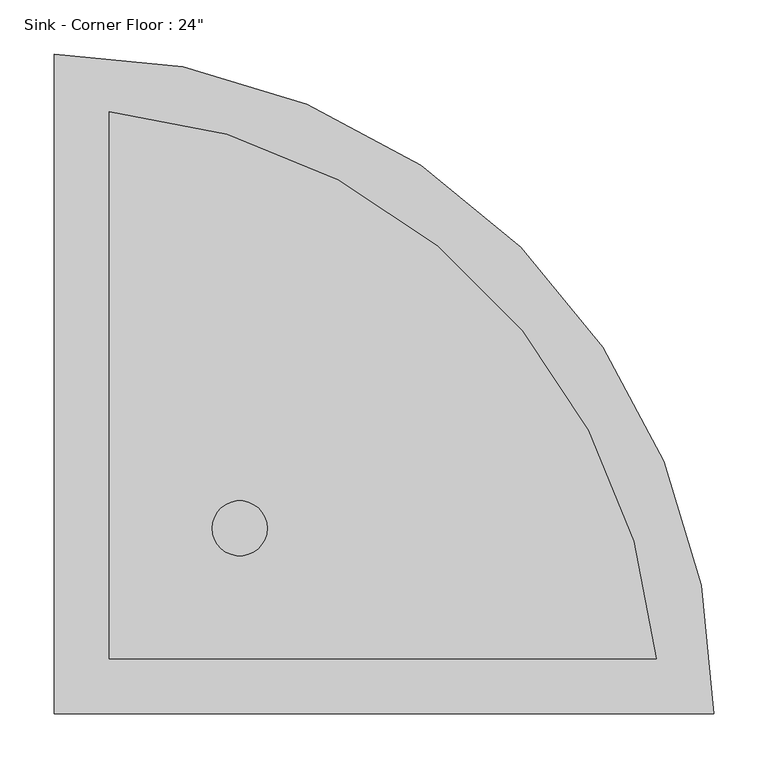
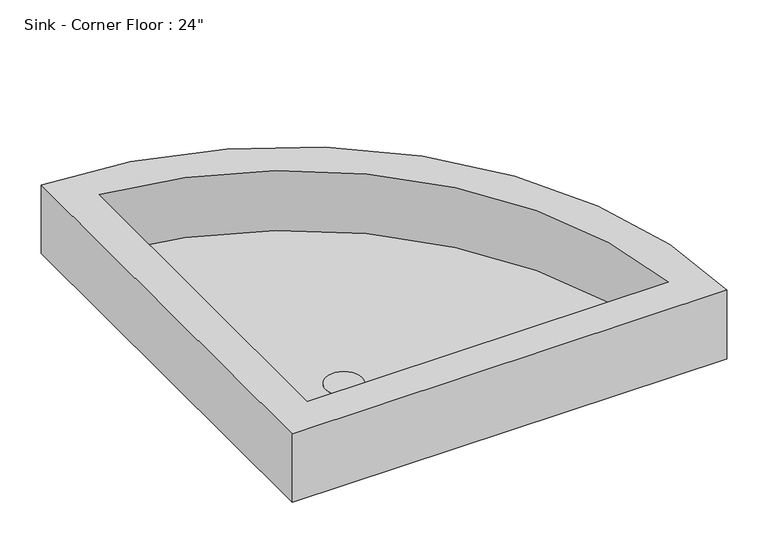
"""IFC4 building model written with IfcOpenShell, lengths in millimetres: flow terminal geometry."""

from ifc_helpers import new_model, si_unit, point, frame, frame_2d, origin, origin_with_axes, place, context, project, spatial, polyline, circle_curve, trimmed, segment, composite_curve, outline, extrude, source, transform, mapped, element, save
from ifc_brep_helpers import plane_surface, cylinder_surface, revolved_surface, advanced_brep


def flow_terminal_bd5cdcf8(model_context):
    return source(origin(), model_context, "Body", "SolidModel", [
        extrude(outline(composite_curve([segment(trimmed(circle_curve(frame_2d((171.45, 171.45)), 25.4), [point((146.05, 171.45))], [point((196.85, 171.45))], False, "CARTESIAN"), True, "CONTINUOUS"), segment(trimmed(circle_curve(frame_2d((171.45, 171.45)), 25.4), [point((196.85, 171.45))], [point((146.05, 171.45))], False, "CARTESIAN"), True, "CONTINUOUS")], self_intersect=False)), origin_with_axes(), (0.0, 0.0, 1.0), 12.7),
        advanced_brep(
        [(0.0, 0.0, 101.6), (609.6, 0.0, 101.6), (0.0, 609.6, 101.6), (556.4861184, 50.8, 101.6), (50.8, 50.8, 101.6), (50.8, 556.4861184, 101.6), (0.0, 0.0, 0.0), (0.0, 609.6, 0.0), (609.6, 0.0, 0.0), (50.8, 50.8, 12.7), (556.4861184, 50.8, 12.7), (50.8, 556.4861184, 12.7)],
        [
            (0, 1),
            (1, 2, circle_curve(frame((0.0, 0.0, 101.6), z_axis=(0.0, 0.0, 1.0), x_axis=(1.0, 0.0, 0.0)), 609.6)),
            (2, 0),
            (3, 4),
            (4, 5),
            (5, 3, circle_curve(frame((0.0, 0.0, 101.6), z_axis=(0.0, 0.0, -1.0), x_axis=(1.0, 0.0, 0.0)), 558.8)),
            (6, 7),
            (7, 8, circle_curve(frame((0.0, 0.0, 0.0), z_axis=(0.0, 0.0, -1.0), x_axis=(1.0, 0.0, 0.0)), 609.6)),
            (8, 6),
            (0, 6),
            (8, 1),
            (7, 2),
            (9, 10),
            (10, 11, circle_curve(frame((0.0, 0.0, 12.7), z_axis=(0.0, 0.0, 1.0), x_axis=(1.0, 0.0, 0.0)), 558.8)),
            (11, 9),
            (9, 4),
            (3, 10),
            (5, 11),
        ],
        [
            plane_surface(frame((0.0, 0.0, 101.6), z_axis=(0.0, 0.0, 1.0), x_axis=(1.0, 0.0, 0.0))),
            plane_surface(frame((0.0, 0.0, 0.0), z_axis=(0.0, 0.0, -1.0), x_axis=(-1.0, 0.0, 0.0))),
            plane_surface(frame((0.0, 0.0, 101.6), z_axis=(0.0, -1.0, 0.0), x_axis=(0.0, 0.0, -1.0))),
            cylinder_surface(origin_with_axes(), 609.6),
            plane_surface(frame((0.0, 609.6, 101.6), z_axis=(-1.0, 0.0, 0.0), x_axis=(0.0, 0.0, -1.0))),
            plane_surface(frame((50.8, 50.8, 12.7), z_axis=(0.0, 0.0, 1.0), x_axis=(-1.0, 0.0, 0.0))),
            plane_surface(frame((50.8, 50.8, 101.6), z_axis=(0.0, 1.0, 0.0), x_axis=(0.0, 0.0, -1.0))),
            revolved_surface(polyline([(558.8, 0.0, 101.6), (558.8, 0.0, 12.7)]), (0.0, 0.0, 12.7), (0.0, 0.0, 1.0)),
            plane_surface(frame((50.8, 556.4861184, 101.6), z_axis=(1.0, 0.0, 0.0), x_axis=(0.0, 0.0, -1.0))),
        ],
        [
            (0, [[1, 2, 3], [4, 5, 6]]),
            (1, [[7, 8, 9]]),
            (2, [[-1, 10, -9, 11]]),
            (3, [[-2, -11, -8, 12]]),
            (4, [[-3, -12, -7, -10]]),
            (5, [[13, 14, 15]]),
            (6, [[-13, 16, -4, 17]]),
            (7, [[-14, -17, -6, 18]]),
            (8, [[-15, -18, -5, -16]]),
        ],
    ),
    ])


if __name__ == "__main__":
    model = new_model("IFC4")
    model_context = context("Model", 3, world=origin())
    ifc_project = project(units=[si_unit("LENGTHUNIT", "METRE", prefix="MILLI")], contexts=[model_context])
    site = spatial("IfcSite", under=ifc_project)
    building = spatial("IfcBuilding", under=site)
    placement = place(None, origin())
    flow_terminal_shape = flow_terminal_bd5cdcf8(model_context)
    element("IfcFlowTerminal", 1, ObjectType="Sink - Corner Floor : 24\"", at=placement, inside=building, context=model_context, shape_type="MappedRepresentation", body=[
        mapped(flow_terminal_shape, transform((0.0, 0.0, 0.0), x_axis=(1.0, 0.0, 0.0), y_axis=(0.0, 1.0, 0.0), z_axis=(0.0, 0.0, 1.0))),
    ])
    save(model, "model.ifc")

# Revit data of these elements
# Type "Sink - Corner Floor : 24\""
#   WFU = 2
#   Sink Radius = 2' - 0"
#   Sink Depth = 0' - 3 1/2"
#   Sanitary Radius = 3/4"
#   Sanitary Diameter = 1 1/2"
#   Radius 1 = 1' - 10"
#   Edge Width = 0' - 2"
#   Sink Material = none
#   HWFU = 0
#   Default Elevation = 0
#   CWFU = 0
